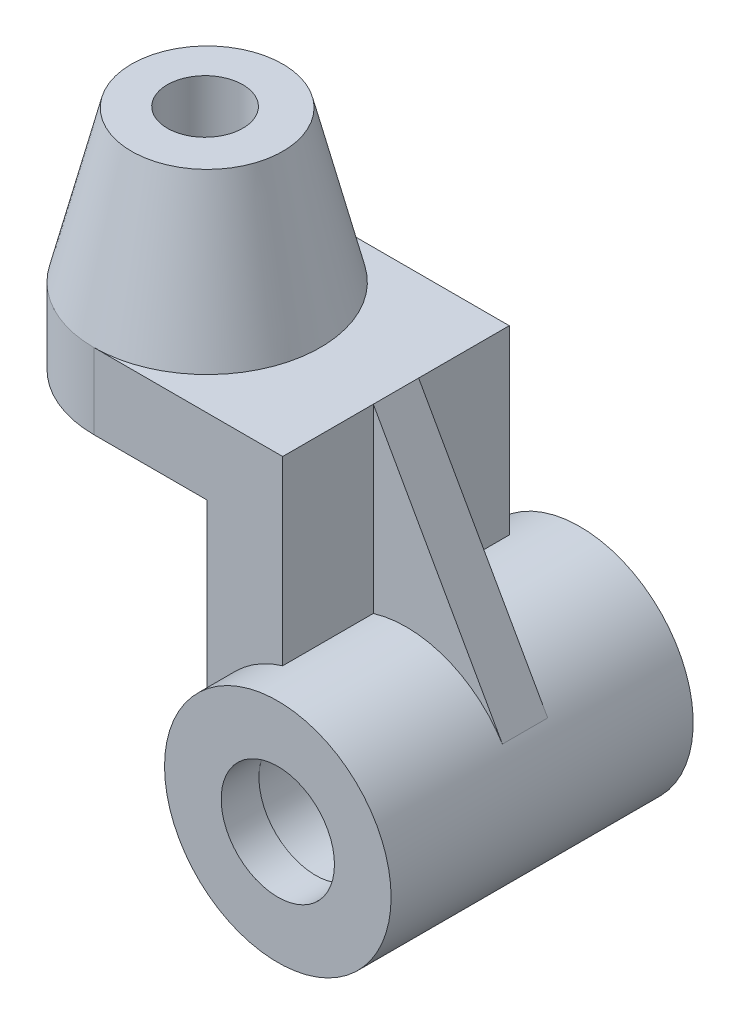
ISO-10303-21;
HEADER;
FILE_DESCRIPTION(('STEP AP214'),'2;1');
FILE_NAME('part.step','',(''),(''),'','','');
FILE_SCHEMA(('AUTOMOTIVE_DESIGN { 1 0 10303 214 1 1 1 1 }'));
ENDSEC;
DATA;
#1=APPLICATION_CONTEXT('core data for automotive mechanical design processes');
#2=APPLICATION_PROTOCOL_DEFINITION('international standard','automotive_design',2000,#1);
#3=PRODUCT_CONTEXT('',#1,'mechanical');
#4=PRODUCT('Part','Part','',(#3));
#5=PRODUCT_RELATED_PRODUCT_CATEGORY('part','',(#4));
#6=PRODUCT_DEFINITION_FORMATION('','',#4);
#7=PRODUCT_DEFINITION_CONTEXT('part definition',#1,'design');
#8=PRODUCT_DEFINITION('design','',#6,#7);
#9=PRODUCT_DEFINITION_SHAPE('','',#8);
#10=(LENGTH_UNIT() NAMED_UNIT(*) SI_UNIT(.MILLI.,.METRE.));
#11=(NAMED_UNIT(*) PLANE_ANGLE_UNIT() SI_UNIT($,.RADIAN.));
#12=(NAMED_UNIT(*) SI_UNIT($,.STERADIAN.) SOLID_ANGLE_UNIT());
#13=UNCERTAINTY_MEASURE_WITH_UNIT(LENGTH_MEASURE(1.E-05),#10,'distance_accuracy_value','');
#14=(GEOMETRIC_REPRESENTATION_CONTEXT(3) GLOBAL_UNCERTAINTY_ASSIGNED_CONTEXT((#13)) GLOBAL_UNIT_ASSIGNED_CONTEXT((#10,
#11,#12)) REPRESENTATION_CONTEXT('',''));
#15=CARTESIAN_POINT('',(0.,0.,0.));
#16=DIRECTION('',(0.,0.,1.));
#17=DIRECTION('',(1.,0.,0.));
#18=AXIS2_PLACEMENT_3D('',#15,#16,#17);
#19=CARTESIAN_POINT('',(0.,76.7082869338697,30.));
#20=DIRECTION('',(0.,-1.,0.));
#21=DIRECTION('',(1.,0.,0.));
#22=AXIS2_PLACEMENT_3D('',#19,#20,#21);
#23=PLANE('',#22);
#24=CARTESIAN_POINT('',(-58.7082869338697,76.7082869338697,0.));
#25=DIRECTION('',(0.,1.,0.));
#26=DIRECTION('',(-1.,0.,0.));
#27=AXIS2_PLACEMENT_3D('',#24,#25,#26);
#28=CIRCLE('',#27,30.);
#29=CARTESIAN_POINT('',(-58.7082869338697,76.7082869338697,30.));
#30=VERTEX_POINT('',#29);
#31=CARTESIAN_POINT('',(-58.7082869338697,76.7082869338697,-30.));
#32=VERTEX_POINT('',#31);
#33=EDGE_CURVE('E142',#30,#32,#28,.T.);
#34=ORIENTED_EDGE('',*,*,#33,.F.);
#35=DIRECTION('',(-1.,0.,0.));
#36=VECTOR('',#35,1.);
#37=CARTESIAN_POINT('',(0.,76.7082869338697,30.));
#38=LINE('',#37,#36);
#39=CARTESIAN_POINT('',(-8.70828693386971,76.7082869338697,30.));
#40=VERTEX_POINT('',#39);
#41=EDGE_CURVE('E109',#40,#30,#38,.T.);
#42=ORIENTED_EDGE('',*,*,#41,.F.);
#43=DIRECTION('',(0.,0.,-1.));
#44=VECTOR('',#43,1.);
#45=CARTESIAN_POINT('',(-8.70828693386971,76.7082869338697,30.));
#46=LINE('',#45,#44);
#47=CARTESIAN_POINT('',(-8.70828693386971,76.7082869338697,6.));
#48=VERTEX_POINT('',#47);
#49=EDGE_CURVE('E112',#40,#48,#46,.T.);
#50=ORIENTED_EDGE('',*,*,#49,.T.);
#51=DIRECTION('',(0.,0.,-1.));
#52=VECTOR('',#51,1.);
#53=CARTESIAN_POINT('',(-8.70828693386971,76.7082869338697,6.));
#54=LINE('',#53,#52);
#55=CARTESIAN_POINT('',(-8.70828693386971,76.7082869338697,-6.));
#56=VERTEX_POINT('',#55);
#57=EDGE_CURVE('E173',#48,#56,#54,.T.);
#58=ORIENTED_EDGE('',*,*,#57,.T.);
#59=CARTESIAN_POINT('',(-8.70828693386971,76.7082869338697,-30.));
#60=VERTEX_POINT('',#59);
#61=EDGE_CURVE('E103',#56,#60,#46,.T.);
#62=ORIENTED_EDGE('',*,*,#61,.T.);
#63=DIRECTION('',(-1.,0.,0.));
#64=VECTOR('',#63,1.);
#65=CARTESIAN_POINT('',(0.,76.7082869338697,-30.));
#66=LINE('',#65,#64);
#67=EDGE_CURVE('E95',#60,#32,#66,.T.);
#68=ORIENTED_EDGE('',*,*,#67,.T.);
#69=EDGE_LOOP('',(#34,#42,#50,#58,#62,#68));
#70=FACE_BOUND('',#69,.T.);
#71=ADVANCED_FACE('F43',(#70),#23,.F.);
#72=CARTESIAN_POINT('',(0.,56.7082869338697,30.));
#73=DIRECTION('',(0.,1.,0.));
#74=DIRECTION('',(0.,0.,1.));
#75=AXIS2_PLACEMENT_3D('',#72,#73,#74);
#76=PLANE('',#75);
#77=CARTESIAN_POINT('',(-59.2629497365909,56.7082869338697,0.));
#78=DIRECTION('',(0.,1.,0.));
#79=DIRECTION('',(0.,0.,1.));
#80=AXIS2_PLACEMENT_3D('',#77,#78,#79);
#81=CIRCLE('',#80,10.);
#82=CARTESIAN_POINT('',(-69.2629497365909,56.7082869338697,0.));
#83=VERTEX_POINT('',#82);
#84=EDGE_CURVE('E128',#83,#83,#81,.T.);
#85=ORIENTED_EDGE('',*,*,#84,.T.);
#86=EDGE_LOOP('',(#85));
#87=FACE_BOUND('',#86,.T.);
#88=CARTESIAN_POINT('',(-58.7082869338697,56.7082869338697,0.));
#89=DIRECTION('',(0.,1.,0.));
#90=DIRECTION('',(0.,0.,1.));
#91=AXIS2_PLACEMENT_3D('',#88,#89,#90);
#92=CIRCLE('',#91,30.);
#93=CARTESIAN_POINT('',(-58.7082869338697,56.7082869338697,-30.));
#94=VERTEX_POINT('',#93);
#95=CARTESIAN_POINT('',(-58.7082869338697,56.7082869338697,30.));
#96=VERTEX_POINT('',#95);
#97=EDGE_CURVE('E11',#94,#96,#92,.T.);
#98=ORIENTED_EDGE('',*,*,#97,.F.);
#99=DIRECTION('',(1.,0.,0.));
#100=VECTOR('',#99,1.);
#101=CARTESIAN_POINT('',(0.,56.7082869338697,-30.));
#102=LINE('',#101,#100);
#103=CARTESIAN_POINT('',(-28.7082869338697,56.7082869338697,-30.));
#104=VERTEX_POINT('',#103);
#105=EDGE_CURVE('E81',#94,#104,#102,.T.);
#106=ORIENTED_EDGE('',*,*,#105,.T.);
#107=DIRECTION('',(0.,0.,-1.));
#108=VECTOR('',#107,1.);
#109=CARTESIAN_POINT('',(-28.7082869338697,56.7082869338697,30.));
#110=LINE('',#109,#108);
#111=CARTESIAN_POINT('',(-28.7082869338697,56.7082869338697,30.));
#112=VERTEX_POINT('',#111);
#113=EDGE_CURVE('E83',#112,#104,#110,.T.);
#114=ORIENTED_EDGE('',*,*,#113,.F.);
#115=DIRECTION('',(1.,0.,0.));
#116=VECTOR('',#115,1.);
#117=CARTESIAN_POINT('',(0.,56.7082869338697,30.));
#118=LINE('',#117,#116);
#119=EDGE_CURVE('E70',#96,#112,#118,.T.);
#120=ORIENTED_EDGE('',*,*,#119,.F.);
#121=EDGE_LOOP('',(#98,#106,#114,#120));
#122=FACE_BOUND('',#121,.T.);
#123=ADVANCED_FACE('F82',(#87,#122),#76,.F.);
#124=CARTESIAN_POINT('',(-8.7082869338697,0.,30.));
#125=DIRECTION('',(1.,0.,0.));
#126=DIRECTION('',(0.,1.,0.));
#127=AXIS2_PLACEMENT_3D('',#124,#125,#126);
#128=PLANE('',#127);
#129=DIRECTION('',(0.,0.,-1.));
#130=VECTOR('',#129,1.);
#131=CARTESIAN_POINT('',(-8.7082869338697,28.7082869338697,20.));
#132=LINE('',#131,#130);
#133=CARTESIAN_POINT('',(-8.7082869338697,28.7082869338697,6.));
#134=VERTEX_POINT('',#133);
#135=CARTESIAN_POINT('',(-8.7082869338697,28.7082869338697,30.));
#136=VERTEX_POINT('',#135);
#137=EDGE_CURVE('E119',#134,#136,#132,.F.);
#138=ORIENTED_EDGE('',*,*,#137,.F.);
#139=DIRECTION('',(0.,-1.,0.));
#140=VECTOR('',#139,1.);
#141=CARTESIAN_POINT('',(-8.70828693386971,76.7082869338697,6.));
#142=LINE('',#141,#140);
#143=EDGE_CURVE('E159',#48,#134,#142,.T.);
#144=ORIENTED_EDGE('',*,*,#143,.F.);
#145=ORIENTED_EDGE('',*,*,#49,.F.);
#146=DIRECTION('',(0.,-1.,0.));
#147=VECTOR('',#146,1.);
#148=CARTESIAN_POINT('',(-8.7082869338697,0.,30.));
#149=LINE('',#148,#147);
#150=EDGE_CURVE('E110',#40,#136,#149,.T.);
#151=ORIENTED_EDGE('',*,*,#150,.T.);
#152=EDGE_LOOP('',(#138,#144,#145,#151));
#153=FACE_BOUND('',#152,.T.);
#154=ADVANCED_FACE('F237',(#153),#128,.T.);
#155=CARTESIAN_POINT('',(0.,0.,20.));
#156=DIRECTION('',(0.,0.,-1.));
#157=DIRECTION('',(-1.,0.,0.));
#158=AXIS2_PLACEMENT_3D('',#155,#156,#157);
#159=CYLINDRICAL_SURFACE('',#158,30.);
#160=CARTESIAN_POINT('',(0.,0.,-40.));
#161=DIRECTION('',(0.,0.,-1.));
#162=DIRECTION('',(-1.,0.,0.));
#163=AXIS2_PLACEMENT_3D('',#160,#161,#162);
#164=CIRCLE('',#163,30.);
#165=CARTESIAN_POINT('',(-30.,0.,-40.));
#166=VERTEX_POINT('',#165);
#167=EDGE_CURVE('E176',#166,#166,#164,.T.);
#168=ORIENTED_EDGE('',*,*,#167,.F.);
#169=EDGE_LOOP('',(#168));
#170=FACE_BOUND('',#169,.T.);
#171=CARTESIAN_POINT('',(0.,0.,40.));
#172=DIRECTION('',(0.,0.,1.));
#173=DIRECTION('',(1.,0.,0.));
#174=AXIS2_PLACEMENT_3D('',#171,#172,#173);
#175=CIRCLE('',#174,30.);
#176=CARTESIAN_POINT('',(30.,0.,40.));
#177=VERTEX_POINT('',#176);
#178=EDGE_CURVE('E182',#177,#177,#175,.T.);
#179=ORIENTED_EDGE('',*,*,#178,.F.);
#180=EDGE_LOOP('',(#179));
#181=FACE_BOUND('',#180,.T.);
#182=CARTESIAN_POINT('',(0.,0.,6.));
#183=DIRECTION('',(0.,0.,-1.));
#184=DIRECTION('',(-1.,0.,0.));
#185=AXIS2_PLACEMENT_3D('',#182,#183,#184);
#186=CIRCLE('',#185,30.0000000000001);
#187=CARTESIAN_POINT('',(25.4774783089231,15.8397632248197,6.));
#188=VERTEX_POINT('',#187);
#189=EDGE_CURVE('E162',#134,#188,#186,.T.);
#190=ORIENTED_EDGE('',*,*,#189,.F.);
#191=ORIENTED_EDGE('',*,*,#137,.T.);
#192=CARTESIAN_POINT('',(0.,0.,30.));
#193=DIRECTION('',(0.,0.,1.));
#194=DIRECTION('',(1.,0.,0.));
#195=AXIS2_PLACEMENT_3D('',#192,#193,#194);
#196=CIRCLE('',#195,30.);
#197=CARTESIAN_POINT('',(-28.7082869338697,8.70828693386971,30.));
#198=VERTEX_POINT('',#197);
#199=EDGE_CURVE('E187',#198,#136,#196,.F.);
#200=ORIENTED_EDGE('',*,*,#199,.F.);
#201=DIRECTION('',(0.,0.,-1.));
#202=VECTOR('',#201,1.);
#203=CARTESIAN_POINT('',(-28.7082869338697,8.7082869338697,20.));
#204=LINE('',#203,#202);
#205=CARTESIAN_POINT('',(-28.7082869338697,8.70828693386971,-30.));
#206=VERTEX_POINT('',#205);
#207=EDGE_CURVE('E120',#198,#206,#204,.T.);
#208=ORIENTED_EDGE('',*,*,#207,.T.);
#209=CARTESIAN_POINT('',(0.,0.,-30.));
#210=DIRECTION('',(0.,0.,1.));
#211=DIRECTION('',(1.,0.,0.));
#212=AXIS2_PLACEMENT_3D('',#209,#210,#211);
#213=CIRCLE('',#212,30.);
#214=CARTESIAN_POINT('',(-8.7082869338697,28.7082869338697,-30.));
#215=VERTEX_POINT('',#214);
#216=EDGE_CURVE('E106',#206,#215,#213,.F.);
#217=ORIENTED_EDGE('',*,*,#216,.T.);
#218=CARTESIAN_POINT('',(-8.7082869338697,28.7082869338697,-6.));
#219=VERTEX_POINT('',#218);
#220=EDGE_CURVE('E51',#215,#219,#132,.F.);
#221=ORIENTED_EDGE('',*,*,#220,.T.);
#222=CARTESIAN_POINT('',(0.,0.,-6.));
#223=DIRECTION('',(0.,0.,-1.));
#224=DIRECTION('',(-1.,0.,0.));
#225=AXIS2_PLACEMENT_3D('',#222,#223,#224);
#226=CIRCLE('',#225,30.0000000000001);
#227=CARTESIAN_POINT('',(25.4774783089231,15.8397632248197,-6.));
#228=VERTEX_POINT('',#227);
#229=EDGE_CURVE('E156',#219,#228,#226,.T.);
#230=ORIENTED_EDGE('',*,*,#229,.T.);
#231=DIRECTION('',(0.,0.,-1.));
#232=VECTOR('',#231,1.);
#233=CARTESIAN_POINT('',(25.4774783089231,15.8397632248197,6.));
#234=LINE('',#233,#232);
#235=EDGE_CURVE('E164',#188,#228,#234,.T.);
#236=ORIENTED_EDGE('',*,*,#235,.F.);
#237=EDGE_LOOP('',(#190,#191,#200,#208,#217,#221,#230,#236));
#238=FACE_BOUND('',#237,.T.);
#239=ADVANCED_FACE('F44',(#170,#181,#238),#159,.T.);
#240=CARTESIAN_POINT('',(0.,0.,-30.));
#241=DIRECTION('',(0.,0.,1.));
#242=DIRECTION('',(1.,0.,0.));
#243=AXIS2_PLACEMENT_3D('',#240,#241,#242);
#244=PLANE('',#243);
#245=ORIENTED_EDGE('',*,*,#105,.F.);
#246=DIRECTION('',(0.,1.,0.));
#247=VECTOR('',#246,1.);
#248=CARTESIAN_POINT('',(-58.7082869338697,36.7082869338697,-30.));
#249=LINE('',#248,#247);
#250=EDGE_CURVE('E150',#94,#32,#249,.T.);
#251=ORIENTED_EDGE('',*,*,#250,.T.);
#252=ORIENTED_EDGE('',*,*,#67,.F.);
#253=DIRECTION('',(0.,-1.,0.));
#254=VECTOR('',#253,1.);
#255=CARTESIAN_POINT('',(-8.7082869338697,0.,-30.));
#256=LINE('',#255,#254);
#257=EDGE_CURVE('E189',#60,#215,#256,.T.);
#258=ORIENTED_EDGE('',*,*,#257,.T.);
#259=ORIENTED_EDGE('',*,*,#216,.F.);
#260=DIRECTION('',(0.,1.,0.));
#261=VECTOR('',#260,1.);
#262=CARTESIAN_POINT('',(-28.7082869338697,0.,-30.));
#263=LINE('',#262,#261);
#264=EDGE_CURVE('E92',#206,#104,#263,.T.);
#265=ORIENTED_EDGE('',*,*,#264,.T.);
#266=EDGE_LOOP('',(#245,#251,#252,#258,#259,#265));
#267=FACE_BOUND('',#266,.T.);
#268=ADVANCED_FACE('F101',(#267),#244,.F.);
#269=CARTESIAN_POINT('',(0.,0.,30.));
#270=DIRECTION('',(0.,0.,1.));
#271=DIRECTION('',(1.,0.,0.));
#272=AXIS2_PLACEMENT_3D('',#269,#270,#271);
#273=PLANE('',#272);
#274=DIRECTION('',(0.,1.,0.));
#275=VECTOR('',#274,1.);
#276=CARTESIAN_POINT('',(-58.7082869338697,36.7082869338697,30.));
#277=LINE('',#276,#275);
#278=EDGE_CURVE('E155',#96,#30,#277,.T.);
#279=ORIENTED_EDGE('',*,*,#278,.F.);
#280=ORIENTED_EDGE('',*,*,#119,.T.);
#281=DIRECTION('',(0.,1.,0.));
#282=VECTOR('',#281,1.);
#283=CARTESIAN_POINT('',(-28.7082869338697,0.,30.));
#284=LINE('',#283,#282);
#285=EDGE_CURVE('E99',#198,#112,#284,.T.);
#286=ORIENTED_EDGE('',*,*,#285,.F.);
#287=ORIENTED_EDGE('',*,*,#199,.T.);
#288=ORIENTED_EDGE('',*,*,#150,.F.);
#289=ORIENTED_EDGE('',*,*,#41,.T.);
#290=EDGE_LOOP('',(#279,#280,#286,#287,#288,#289));
#291=FACE_BOUND('',#290,.T.);
#292=ADVANCED_FACE('F211',(#291),#273,.T.);
#293=CARTESIAN_POINT('',(-28.7082869338697,0.,30.));
#294=DIRECTION('',(-1.,0.,0.));
#295=DIRECTION('',(0.,0.,1.));
#296=AXIS2_PLACEMENT_3D('',#293,#294,#295);
#297=PLANE('',#296);
#298=ORIENTED_EDGE('',*,*,#264,.F.);
#299=ORIENTED_EDGE('',*,*,#207,.F.);
#300=ORIENTED_EDGE('',*,*,#285,.T.);
#301=ORIENTED_EDGE('',*,*,#113,.T.);
#302=EDGE_LOOP('',(#298,#299,#300,#301));
#303=FACE_BOUND('',#302,.T.);
#304=ADVANCED_FACE('F98',(#303),#297,.T.);
#305=DIRECTION('',(0.,-1.,0.));
#306=VECTOR('',#305,1.);
#307=CARTESIAN_POINT('',(-8.70828693386971,76.7082869338697,-6.));
#308=LINE('',#307,#306);
#309=EDGE_CURVE('E170',#56,#219,#308,.T.);
#310=ORIENTED_EDGE('',*,*,#309,.T.);
#311=ORIENTED_EDGE('',*,*,#220,.F.);
#312=ORIENTED_EDGE('',*,*,#257,.F.);
#313=ORIENTED_EDGE('',*,*,#61,.F.);
#314=EDGE_LOOP('',(#310,#311,#312,#313));
#315=FACE_BOUND('',#314,.T.);
#316=ADVANCED_FACE('F244',(#315),#128,.T.);
#317=CARTESIAN_POINT('',(0.,0.,40.));
#318=DIRECTION('',(0.,0.,1.));
#319=DIRECTION('',(1.,0.,0.));
#320=AXIS2_PLACEMENT_3D('',#317,#318,#319);
#321=PLANE('',#320);
#322=ORIENTED_EDGE('',*,*,#178,.T.);
#323=EDGE_LOOP('',(#322));
#324=FACE_BOUND('',#323,.T.);
#325=CARTESIAN_POINT('',(0.,0.,40.));
#326=DIRECTION('',(0.,0.,1.));
#327=DIRECTION('',(1.,0.,0.));
#328=AXIS2_PLACEMENT_3D('',#325,#326,#327);
#329=CIRCLE('',#328,15.);
#330=CARTESIAN_POINT('',(15.,0.,40.));
#331=VERTEX_POINT('',#330);
#332=EDGE_CURVE('E179',#331,#331,#329,.T.);
#333=ORIENTED_EDGE('',*,*,#332,.F.);
#334=EDGE_LOOP('',(#333));
#335=FACE_BOUND('',#334,.T.);
#336=ADVANCED_FACE('F266',(#324,#335),#321,.T.);
#337=CARTESIAN_POINT('',(0.,0.,40.));
#338=DIRECTION('',(0.,0.,-1.));
#339=DIRECTION('',(-1.,0.,0.));
#340=AXIS2_PLACEMENT_3D('',#337,#338,#339);
#341=CYLINDRICAL_SURFACE('',#340,15.);
#342=CARTESIAN_POINT('',(0.,0.,30.));
#343=DIRECTION('',(0.,0.,1.));
#344=DIRECTION('',(1.,0.,0.));
#345=AXIS2_PLACEMENT_3D('',#342,#343,#344);
#346=CIRCLE('',#345,15.);
#347=CARTESIAN_POINT('',(15.,0.,30.));
#348=VERTEX_POINT('',#347);
#349=EDGE_CURVE('E125',#348,#348,#346,.F.);
#350=ORIENTED_EDGE('',*,*,#349,.T.);
#351=EDGE_LOOP('',(#350));
#352=FACE_BOUND('',#351,.T.);
#353=ORIENTED_EDGE('',*,*,#332,.T.);
#354=EDGE_LOOP('',(#353));
#355=FACE_BOUND('',#354,.T.);
#356=ADVANCED_FACE('F273',(#352,#355),#341,.F.);
#357=CARTESIAN_POINT('',(0.,0.,-40.));
#358=DIRECTION('',(0.,0.,-1.));
#359=DIRECTION('',(-1.,0.,0.));
#360=AXIS2_PLACEMENT_3D('',#357,#358,#359);
#361=PLANE('',#360);
#362=CARTESIAN_POINT('',(0.,0.,-40.));
#363=DIRECTION('',(0.,0.,1.));
#364=DIRECTION('',(1.,0.,0.));
#365=AXIS2_PLACEMENT_3D('',#362,#363,#364);
#366=CIRCLE('',#365,15.3089268479194);
#367=CARTESIAN_POINT('',(15.3089268479194,0.,-40.));
#368=VERTEX_POINT('',#367);
#369=EDGE_CURVE('E123',#368,#368,#366,.T.);
#370=ORIENTED_EDGE('',*,*,#369,.T.);
#371=EDGE_LOOP('',(#370));
#372=FACE_BOUND('',#371,.T.);
#373=ORIENTED_EDGE('',*,*,#167,.T.);
#374=EDGE_LOOP('',(#373));
#375=FACE_BOUND('',#374,.T.);
#376=ADVANCED_FACE('F291',(#372,#375),#361,.T.);
#377=CARTESIAN_POINT('',(-8.70828693386971,76.7082869338697,6.));
#378=DIRECTION('',(-0.871898397864155,-0.489686822164861,0.));
#379=DIRECTION('',(0.489686822164861,-0.871898397864155,0.));
#380=AXIS2_PLACEMENT_3D('',#377,#378,#379);
#381=PLANE('',#380);
#382=DIRECTION('',(-0.489686822164861,0.871898397864155,0.));
#383=VECTOR('',#382,1.);
#384=CARTESIAN_POINT('',(-8.70828693386971,76.7082869338697,-6.));
#385=LINE('',#384,#383);
#386=EDGE_CURVE('E59',#228,#56,#385,.T.);
#387=ORIENTED_EDGE('',*,*,#386,.T.);
#388=ORIENTED_EDGE('',*,*,#57,.F.);
#389=DIRECTION('',(-0.489686822164861,0.871898397864155,0.));
#390=VECTOR('',#389,1.);
#391=CARTESIAN_POINT('',(-8.70828693386971,76.7082869338697,6.));
#392=LINE('',#391,#390);
#393=EDGE_CURVE('E153',#188,#48,#392,.T.);
#394=ORIENTED_EDGE('',*,*,#393,.F.);
#395=ORIENTED_EDGE('',*,*,#235,.T.);
#396=EDGE_LOOP('',(#387,#388,#394,#395));
#397=FACE_BOUND('',#396,.T.);
#398=ADVANCED_FACE('F243',(#397),#381,.F.);
#399=CARTESIAN_POINT('',(0.,0.,6.));
#400=DIRECTION('',(0.,0.,-1.));
#401=DIRECTION('',(-1.,0.,0.));
#402=AXIS2_PLACEMENT_3D('',#399,#400,#401);
#403=PLANE('',#402);
#404=ORIENTED_EDGE('',*,*,#393,.T.);
#405=ORIENTED_EDGE('',*,*,#143,.T.);
#406=ORIENTED_EDGE('',*,*,#189,.T.);
#407=EDGE_LOOP('',(#404,#405,#406));
#408=FACE_BOUND('',#407,.T.);
#409=ADVANCED_FACE('F247',(#408),#403,.F.);
#410=CARTESIAN_POINT('',(0.,0.,-6.));
#411=DIRECTION('',(0.,0.,-1.));
#412=DIRECTION('',(-1.,0.,0.));
#413=AXIS2_PLACEMENT_3D('',#410,#411,#412);
#414=PLANE('',#413);
#415=ORIENTED_EDGE('',*,*,#386,.F.);
#416=ORIENTED_EDGE('',*,*,#229,.F.);
#417=ORIENTED_EDGE('',*,*,#309,.F.);
#418=EDGE_LOOP('',(#415,#416,#417));
#419=FACE_BOUND('',#418,.T.);
#420=ADVANCED_FACE('F246',(#419),#414,.T.);
#421=CARTESIAN_POINT('',(-58.7082869338697,36.7082869338697,0.));
#422=DIRECTION('',(0.,1.,0.));
#423=DIRECTION('',(-1.,0.,0.));
#424=AXIS2_PLACEMENT_3D('',#421,#422,#423);
#425=CYLINDRICAL_SURFACE('',#424,30.);
#426=ORIENTED_EDGE('',*,*,#97,.T.);
#427=ORIENTED_EDGE('',*,*,#278,.T.);
#428=CARTESIAN_POINT('',(-58.7082869338697,76.7082869338697,0.));
#429=DIRECTION('',(0.,1.,0.));
#430=DIRECTION('',(-1.,0.,0.));
#431=AXIS2_PLACEMENT_3D('',#428,#429,#430);
#432=CIRCLE('',#431,30.);
#433=EDGE_CURVE('E148',#32,#30,#432,.T.);
#434=ORIENTED_EDGE('',*,*,#433,.F.);
#435=ORIENTED_EDGE('',*,*,#250,.F.);
#436=EDGE_LOOP('',(#426,#427,#434,#435));
#437=FACE_BOUND('',#436,.T.);
#438=ADVANCED_FACE('F209',(#437),#425,.T.);
#439=CARTESIAN_POINT('',(-58.7082869338697,76.7082869338697,0.));
#440=DIRECTION('',(0.,-1.,0.));
#441=DIRECTION('',(-1.,0.,0.));
#442=AXIS2_PLACEMENT_3D('',#439,#440,#441);
#443=CONICAL_SURFACE('',#442,30.,0.244346095279207);
#444=CARTESIAN_POINT('',(-58.7082869338697,116.70828693387,0.));
#445=DIRECTION('',(0.,1.,0.));
#446=DIRECTION('',(-1.,0.,0.));
#447=AXIS2_PLACEMENT_3D('',#444,#445,#446);
#448=CIRCLE('',#447,20.0268798862728);
#449=CARTESIAN_POINT('',(-78.7351668201425,116.70828693387,0.));
#450=VERTEX_POINT('',#449);
#451=EDGE_CURVE('E144',#450,#450,#448,.T.);
#452=ORIENTED_EDGE('',*,*,#451,.F.);
#453=EDGE_LOOP('',(#452));
#454=FACE_BOUND('',#453,.T.);
#455=ORIENTED_EDGE('',*,*,#33,.T.);
#456=ORIENTED_EDGE('',*,*,#433,.T.);
#457=EDGE_LOOP('',(#455,#456));
#458=FACE_BOUND('',#457,.T.);
#459=ADVANCED_FACE('F207',(#454,#458),#443,.T.);
#460=CARTESIAN_POINT('',(-58.7082869338697,116.70828693387,0.));
#461=DIRECTION('',(0.,1.,0.));
#462=DIRECTION('',(-1.,0.,0.));
#463=AXIS2_PLACEMENT_3D('',#460,#461,#462);
#464=PLANE('',#463);
#465=CARTESIAN_POINT('',(-59.2629497365909,116.70828693387,0.));
#466=DIRECTION('',(0.,1.,0.));
#467=DIRECTION('',(-1.,0.,0.));
#468=AXIS2_PLACEMENT_3D('',#465,#466,#467);
#469=CIRCLE('',#468,10.);
#470=CARTESIAN_POINT('',(-69.2629497365909,116.70828693387,0.));
#471=VERTEX_POINT('',#470);
#472=EDGE_CURVE('E121',#471,#471,#469,.T.);
#473=ORIENTED_EDGE('',*,*,#472,.F.);
#474=EDGE_LOOP('',(#473));
#475=FACE_BOUND('',#474,.T.);
#476=ORIENTED_EDGE('',*,*,#451,.T.);
#477=EDGE_LOOP('',(#476));
#478=FACE_BOUND('',#477,.T.);
#479=ADVANCED_FACE('F400',(#475,#478),#464,.T.);
#480=CARTESIAN_POINT('',(-59.2629497365909,-30.,0.));
#481=DIRECTION('',(0.,1.,0.));
#482=DIRECTION('',(-1.,0.,0.));
#483=AXIS2_PLACEMENT_3D('',#480,#481,#482);
#484=CYLINDRICAL_SURFACE('',#483,10.);
#485=CARTESIAN_POINT('',(-69.2629497365909,116.70828693387,0.));
#486=CARTESIAN_POINT('',(-69.2629497365909,116.08328693387,0.));
#487=CARTESIAN_POINT('',(-69.2629497365909,115.45828693387,0.));
#488=CARTESIAN_POINT('',(-69.2629497365909,114.20828693387,0.));
#489=CARTESIAN_POINT('',(-69.2629497365909,113.58328693387,0.));
#490=CARTESIAN_POINT('',(-69.2629497365909,112.33328693387,0.));
#491=CARTESIAN_POINT('',(-69.2629497365909,111.70828693387,0.));
#492=CARTESIAN_POINT('',(-69.2629497365909,110.45828693387,0.));
#493=CARTESIAN_POINT('',(-69.2629497365909,109.83328693387,0.));
#494=CARTESIAN_POINT('',(-69.2629497365909,108.58328693387,0.));
#495=CARTESIAN_POINT('',(-69.2629497365909,107.95828693387,0.));
#496=CARTESIAN_POINT('',(-69.2629497365909,106.70828693387,0.));
#497=CARTESIAN_POINT('',(-69.2629497365909,106.08328693387,0.));
#498=CARTESIAN_POINT('',(-69.2629497365909,104.83328693387,0.));
#499=CARTESIAN_POINT('',(-69.2629497365909,104.20828693387,0.));
#500=CARTESIAN_POINT('',(-69.2629497365909,102.95828693387,0.));
#501=CARTESIAN_POINT('',(-69.2629497365909,102.33328693387,0.));
#502=CARTESIAN_POINT('',(-69.2629497365909,101.08328693387,0.));
#503=CARTESIAN_POINT('',(-69.2629497365909,100.45828693387,0.));
#504=CARTESIAN_POINT('',(-69.2629497365909,99.2082869338697,0.));
#505=CARTESIAN_POINT('',(-69.2629497365909,98.5832869338697,0.));
#506=CARTESIAN_POINT('',(-69.2629497365909,97.3332869338697,0.));
#507=CARTESIAN_POINT('',(-69.2629497365909,96.7082869338697,0.));
#508=CARTESIAN_POINT('',(-69.2629497365909,95.4582869338697,0.));
#509=CARTESIAN_POINT('',(-69.2629497365909,94.8332869338697,0.));
#510=CARTESIAN_POINT('',(-69.2629497365909,93.5832869338697,0.));
#511=CARTESIAN_POINT('',(-69.2629497365909,92.9582869338697,0.));
#512=CARTESIAN_POINT('',(-69.2629497365909,91.7082869338697,0.));
#513=CARTESIAN_POINT('',(-69.2629497365909,91.0832869338697,0.));
#514=CARTESIAN_POINT('',(-69.2629497365909,89.8332869338697,0.));
#515=CARTESIAN_POINT('',(-69.2629497365909,89.2082869338697,0.));
#516=CARTESIAN_POINT('',(-69.2629497365909,87.9582869338697,0.));
#517=CARTESIAN_POINT('',(-69.2629497365909,87.3332869338697,0.));
#518=CARTESIAN_POINT('',(-69.2629497365909,86.0832869338697,0.));
#519=CARTESIAN_POINT('',(-69.2629497365909,85.4582869338697,0.));
#520=CARTESIAN_POINT('',(-69.2629497365909,84.2082869338697,0.));
#521=CARTESIAN_POINT('',(-69.2629497365909,83.5832869338697,0.));
#522=CARTESIAN_POINT('',(-69.2629497365909,82.3332869338697,0.));
#523=CARTESIAN_POINT('',(-69.2629497365909,81.7082869338697,0.));
#524=CARTESIAN_POINT('',(-69.2629497365909,80.4582869338697,0.));
#525=CARTESIAN_POINT('',(-69.2629497365909,79.8332869338697,0.));
#526=CARTESIAN_POINT('',(-69.2629497365909,78.5832869338697,0.));
#527=CARTESIAN_POINT('',(-69.2629497365909,77.9582869338697,0.));
#528=CARTESIAN_POINT('',(-69.2629497365909,76.7082869338697,0.));
#529=CARTESIAN_POINT('',(-69.2629497365909,76.0832869338697,0.));
#530=CARTESIAN_POINT('',(-69.2629497365909,74.8332869338697,0.));
#531=CARTESIAN_POINT('',(-69.2629497365909,74.2082869338697,0.));
#532=CARTESIAN_POINT('',(-69.2629497365909,72.9582869338697,0.));
#533=CARTESIAN_POINT('',(-69.2629497365909,72.3332869338697,0.));
#534=CARTESIAN_POINT('',(-69.2629497365909,71.0832869338697,0.));
#535=CARTESIAN_POINT('',(-69.2629497365909,70.4582869338697,0.));
#536=CARTESIAN_POINT('',(-69.2629497365909,69.2082869338697,0.));
#537=CARTESIAN_POINT('',(-69.2629497365909,68.5832869338697,0.));
#538=CARTESIAN_POINT('',(-69.2629497365909,67.3332869338697,0.));
#539=CARTESIAN_POINT('',(-69.2629497365909,66.7082869338697,0.));
#540=CARTESIAN_POINT('',(-69.2629497365909,65.4582869338697,0.));
#541=CARTESIAN_POINT('',(-69.2629497365909,64.8332869338697,0.));
#542=CARTESIAN_POINT('',(-69.2629497365909,63.5832869338697,0.));
#543=CARTESIAN_POINT('',(-69.2629497365909,62.9582869338697,0.));
#544=CARTESIAN_POINT('',(-69.2629497365909,61.7082869338697,0.));
#545=CARTESIAN_POINT('',(-69.2629497365909,61.0832869338697,0.));
#546=CARTESIAN_POINT('',(-69.2629497365909,59.8332869338697,0.));
#547=CARTESIAN_POINT('',(-69.2629497365909,59.2082869338697,0.));
#548=CARTESIAN_POINT('',(-69.2629497365909,57.9582869338697,0.));
#549=CARTESIAN_POINT('',(-69.2629497365909,57.3332869338697,0.));
#550=CARTESIAN_POINT('',(-69.2629497365909,56.7082869338697,0.));
#551=B_SPLINE_CURVE_WITH_KNOTS('',3,(#485,#486,#487,#488,#489,#490,#491,#492,#493,#494,#495,
#496,#497,#498,#499,#500,#501,#502,#503,#504,#505,#506,#507,#508,#509,#510,#511,#512,#513,#514,
#515,#516,#517,#518,#519,#520,#521,#522,#523,#524,#525,#526,#527,#528,#529,#530,#531,#532,#533,
#534,#535,#536,#537,#538,#539,#540,#541,#542,#543,#544,#545,#546,#547,#548,#549,#550),
.UNSPECIFIED.,.F.,.F.,(4,2,2,2,2,2,2,2,2,2,2,2,2,2,2,2,2,2,2,2,2,2,2,2,2,2,2,2,2,2,2,2,4),(0.,
1.87499999999999,3.75,5.62499999999999,7.50000000000001,9.37499999999999,11.25,13.125,15.,
16.875,18.75,20.625,22.5,24.375,26.25,28.125,30.,31.875,33.75,35.625,37.5,39.375,41.25,43.125,
45.,46.875,48.75,50.625,52.5,54.375,56.25,58.125,60.),.UNSPECIFIED.);
#552=EDGE_CURVE('BSEAM406',#471,#83,#551,.T.);
#553=ORIENTED_EDGE('',*,*,#472,.T.);
#554=ORIENTED_EDGE('',*,*,#84,.F.);
#555=ORIENTED_EDGE('',*,*,#552,.T.);
#556=ORIENTED_EDGE('',*,*,#552,.F.);
#557=EDGE_LOOP('',(#553,#555,#554,#556));
#558=FACE_BOUND('',#557,.T.);
#559=ADVANCED_FACE('F406',(#558),#484,.F.);
#560=CARTESIAN_POINT('',(0.,0.,30.));
#561=DIRECTION('',(0.,0.,1.));
#562=DIRECTION('',(1.,0.,0.));
#563=AXIS2_PLACEMENT_3D('',#560,#561,#562);
#564=PLANE('',#563);
#565=CARTESIAN_POINT('',(0.,0.,30.));
#566=DIRECTION('',(0.,0.,1.));
#567=DIRECTION('',(1.,0.,0.));
#568=AXIS2_PLACEMENT_3D('',#565,#566,#567);
#569=CIRCLE('',#568,15.3089268479194);
#570=CARTESIAN_POINT('',(15.3089268479194,0.,30.));
#571=VERTEX_POINT('',#570);
#572=EDGE_CURVE('E135',#571,#571,#569,.T.);
#573=ORIENTED_EDGE('',*,*,#572,.F.);
#574=EDGE_LOOP('',(#573));
#575=FACE_BOUND('',#574,.T.);
#576=ORIENTED_EDGE('',*,*,#349,.F.);
#577=EDGE_LOOP('',(#576));
#578=FACE_BOUND('',#577,.T.);
#579=ADVANCED_FACE('F413',(#575,#578),#564,.F.);
#580=CARTESIAN_POINT('',(0.,0.,-40.));
#581=DIRECTION('',(0.,0.,1.));
#582=DIRECTION('',(1.,0.,0.));
#583=AXIS2_PLACEMENT_3D('',#580,#581,#582);
#584=CYLINDRICAL_SURFACE('',#583,15.3089268479194);
#585=ORIENTED_EDGE('',*,*,#369,.F.);
#586=EDGE_LOOP('',(#585));
#587=FACE_BOUND('',#586,.T.);
#588=ORIENTED_EDGE('',*,*,#572,.T.);
#589=EDGE_LOOP('',(#588));
#590=FACE_BOUND('',#589,.T.);
#591=ADVANCED_FACE('F425',(#587,#590),#584,.F.);
#592=CLOSED_SHELL('',(#71,#123,#154,#239,#268,#292,#304,#316,#336,#356,#376,#398,#409,#420,#438,
#459,#479,#559,#579,#591));
#593=MANIFOLD_SOLID_BREP('B2',#592);
#594=ADVANCED_BREP_SHAPE_REPRESENTATION('',(#18,#593),#14);
#595=SHAPE_DEFINITION_REPRESENTATION(#9,#594);
ENDSEC;
END-ISO-10303-21;
